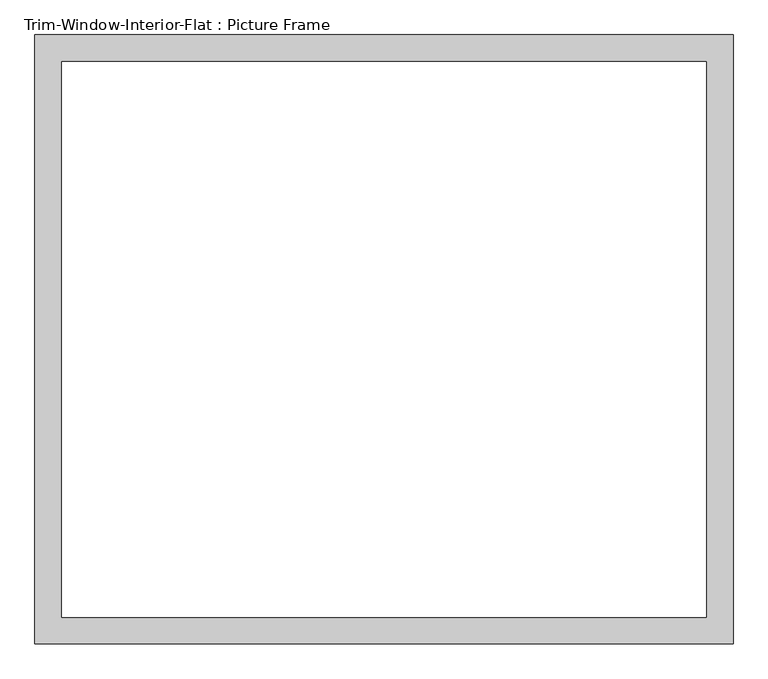
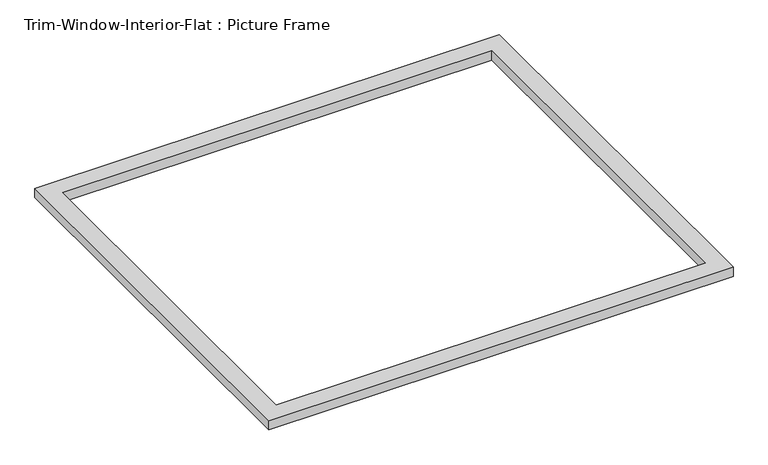
"""IFC4 building model written with IfcOpenShell, lengths in millimetres: proxy geometry, Trim-Window-Interior-Flat : Picture Frame."""

from ifc_helpers import new_model, si_unit, origin, origin_with_axes, place, context, project, spatial, polyline, outline, extrude, source, transform, mapped, element, save


def trim_window_interior_flat_picture_frame_9050e5f4(model_context):
    return source(origin(), model_context, "Body", "SweptSolid", [
        extrude(outline(polyline([(749.3, 44.45), (749.3, -1263.65), (-749.3, -1263.65), (-749.3, 44.45), (749.3, 44.45)]), holes=[polyline([(692.15, -12.7), (-692.15, -12.7), (-692.15, -1206.5), (692.15, -1206.5), (692.15, -12.7)])]), origin_with_axes(), (0.0, 0.0, 1.0), 31.75),
    ])


if __name__ == "__main__":
    model = new_model("IFC4")
    model_context = context("Model", 3, world=origin())
    ifc_project = project(units=[si_unit("LENGTHUNIT", "METRE", prefix="MILLI")], contexts=[model_context])
    site = spatial("IfcSite", under=ifc_project)
    building = spatial("IfcBuilding", under=site)
    placement = place(None, origin())
    trim_window_interior_flat_picture_frame_shape = trim_window_interior_flat_picture_frame_9050e5f4(model_context)
    element("IfcBuildingElementProxy", 1, Name="Trim-Window-Interior-Flat : Picture Frame", ObjectType="Trim-Window-Interior-Flat : Picture Frame", at=placement, inside=building, context=model_context, shape_type="MappedRepresentation", body=[
        mapped(trim_window_interior_flat_picture_frame_shape, transform((0.0, 0.0, 0.0), x_axis=(1.0, 0.0, 0.0), y_axis=(0.0, 1.0, 0.0), z_axis=(0.0, 0.0, 1.0))),
    ])
    save(model, "model.ifc")

# Revit data of these elements
# Type "Trim-Window-Interior-Flat : Picture Frame"
#   Trim Thickness_Picture Frame = 0' - 1 1/4"
#   Trim Width = 0' - 2 1/4"
#   Trim Thickness_with Sill = 0' - 0 3/4"
#   Sill Thickness = 0' - 1 1/4"
#   Opening Width [instance default] = 2' - 0"
#   Opening Height [instance default] = 3' - 0"
#   Default Elevation = 4' - 0"
#   Sill = no
#   Picture Frame = yes
#   Trim Material [instance default] = none
# Element 1 (IfcBuildingElementProxy, "Trim-Window-Interior-Flat : Picture Frame")
#   Opening Width = 4' - 7 1/2"
#   Opening Height = 4' - 0"
#   Trim Material = Wood - Stained
#   Materials on its faces: "Wood - Stained"
# Materials
#   "Wood - Stained": class "Wood", colour RGB 224 178 126, transparency 0, Cost = 0
